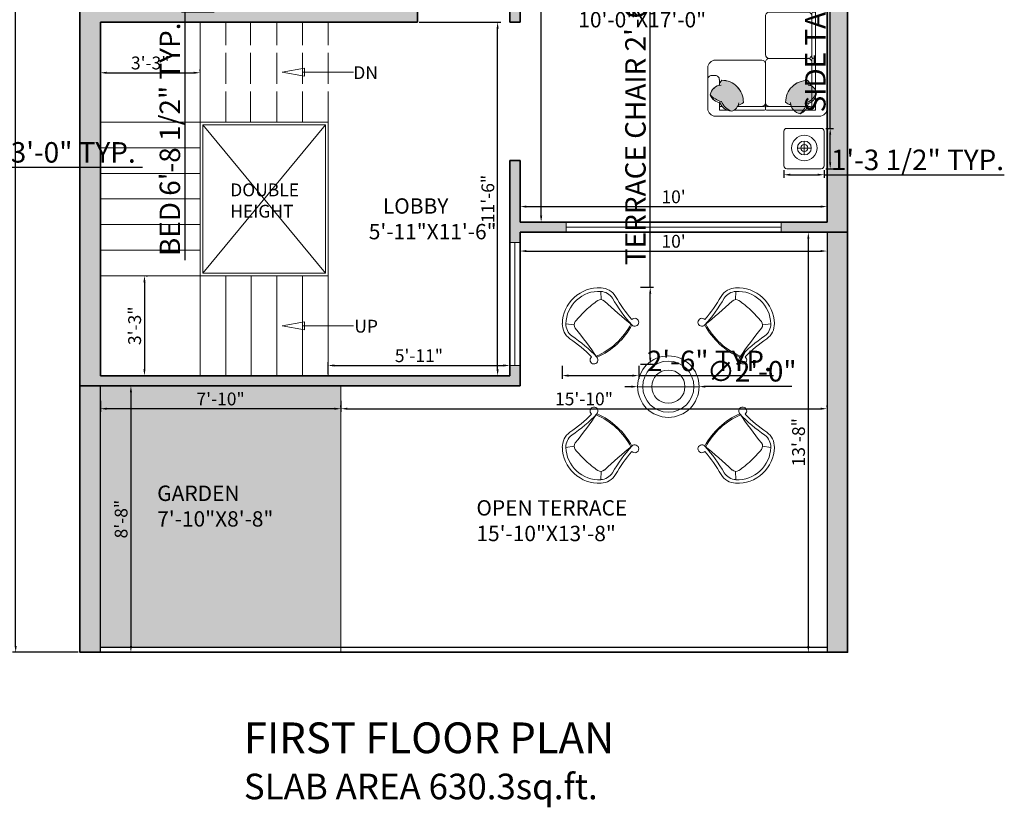
# Model space of a CAD drawing. Units: inches. Extents: x 3259 to 4981, y 1402 to 2026.
# Tile 5 of 11: x 3644 to 4029, y 1415 to 1722. Entities that reach past the tile are written whole.
import ezdxf

# ---------------------------------------------------------------- set-up
doc = ezdxf.new("R2010")
doc.units = ezdxf.units.IN
doc.linetypes.add('ACAD_ISO02W100', pattern=[15, 12, -3])
for name, color, linetype, lineweight in [('A-ANNO-DIMS', 2, 'Continuous', 13), ('A-ANNO-SYMB', 7, 'Continuous', 13), ('A-ANNO-TITL', 7, 'Continuous', 25), ('A-AREA-IDEN', 7, 'Continuous', 18), ('A-DOOR', 3, 'Continuous', 18), ('A-FLOR-STRS', 7, 'Continuous', 18), ('A-FLOR-STRS-OVHD', 8, 'ACAD_ISO02W100', 13), ('A-FURN', 8, 'Continuous', 13), ('A-GLAZ', 4, 'Continuous', 18), ('A-WALL', 7, 'Continuous', 35), ('A-WALL-PATT', 252, 'Continuous', 13), ('A-WALL-PRPT', 7, 'Continuous', 25), ('L-PLNT', 3, 'Continuous', 18)]:
    doc.layers.add(name, color=color, linetype=linetype, lineweight=lineweight)
doc.layers.add('A-WALL-PRPT-PATT', color=9, linetype='Continuous', lineweight=13, true_color=0xc7c8ca)
doc.layers.add('L-PLNT-PATT', color=114, linetype='Continuous', lineweight=13, true_color=0x139b48)
doc.styles.get("Standard").update_dxf_attribs({"font": 'arial.ttf'})
doc.dimstyles.new('ISO-25', dxfattribs={"dimtxt": 8, "dimasz": 2.5, "dimexe": 1.25, "dimexo": 0.625, "dimtad": 1, "dimdec": 1, "dimlunit": 3, "dimtxsty": 'Standard', "dimcen": 2.5, "dimclrd": 4, "dimclre": 4, "dimclrt": 1, "dimadec": 0, "dimazin": 0, "dimtfac": 1, "dimtdec": 1, "dimtmove": 0, "dimatfit": 3, "dimfxl": 1, "dimarcsym": 0})

# ---------------------------------------------------------------- blocks, each defined once
blk = doc.blocks.new('SOFA 1')
at = {"transparency": 33554687}
h = blk.add_hatch(color=256, dxfattribs=at)
h.dxf.hatch_style = 1
h.paths.add_polyline_path([(3769.65, 1307.6, 0.084911), (3767.15, 1309.12, 0.046133), (3766.46, 1311.13), (3759.18, 1311.13, 0.039409), (3758.92, 1310.24, 0.165523), (3756.31, 1309.02, 0.42585), (3767.59, 1297.95, 0.121928), (3769.15, 1300.58, 0.027403), (3769.65, 1300.83)])
h.paths.add_polyline_path([(3765.34, 1313.08), (3760.4, 1313.08, 0.097704), (3759.18, 1311.13), (3766.46, 1311.13, 0.04873)])
h.paths.add_polyline_path([(3763.76, 1314.88, 0.16488), (3760.4, 1313.08), (3765.34, 1313.08, 0.051917)])
h.paths.add_polyline_path([(3771.6, 1305.17, 0.090388), (3769.65, 1307.6), (3769.65, 1300.83, 0.136035), (3771.6, 1302.77)])
h = blk.add_hatch(color=256, dxfattribs=at)
h.dxf.hatch_style = 1
h.paths.add_polyline_path([(3723.52, 1308.63, 0.147724), (3717.76, 1305.24, 0.310469), (3722.42, 1300.4), (3722.42, 1300.25, 0.156703), (3723.62, 1297.8, 0.425821), (3734.69, 1309.08, 0.121928), (3732.05, 1310.63, 0.233216), (3728.6, 1313.59, 0.213835)])
h = blk.add_hatch(color=256, dxfattribs=at)
h.dxf.hatch_style = 1
h.paths.add_polyline_path([(3769.16, 1235.96, 0.122267), (3767.6, 1238.61, 0.425972), (3756.32, 1227.54, 0.165563), (3758.93, 1226.32, 0.309481), (3763.76, 1221.69, 0.002677), (3763.83, 1221.72, 0.146094), (3767.16, 1227.43, 0.212433), (3772.1, 1232.48, 0.235342)])
h = blk.add_hatch(color=256, dxfattribs=at)
h.dxf.hatch_style = 1
h.paths.add_polyline_path([(3769.16, 1225.36, 0.122267), (3767.6, 1228.01, 0.425972), (3756.32, 1216.94, 0.165563), (3758.93, 1215.72, 0.309481), (3763.76, 1211.09, 0.002677), (3763.83, 1211.12, 0.146094), (3767.16, 1216.83, 0.212433), (3772.1, 1221.88, 0.235342)])
for p, q in [((3720.45, 1316.13), (3773.58, 1316.13)), ((3777.51, 1312.19), (3777.51, 1213.72))]:
    blk.add_line(p, q, dxfattribs=at)
for points in [[(3763.76, 1314.88, -0.147724), (3767.15, 1309.12, -0.213355), (3772.1, 1304.05, 0.213355), (3767.15, 1309.12, 0.147724), (3763.76, 1314.88, -0.249545), (3767.86, 1309.77, 0.249545), (3763.77, 1314.89, 0.356779), (3758.8, 1309.23, -0.356779), (3763.76, 1314.88)], [(3717.76, 1305.24, -0.147724), (3723.52, 1308.63, -0.213355), (3728.59, 1313.59, 0.213355), (3723.52, 1308.63, 0.147724), (3717.76, 1305.24, -0.249545), (3722.86, 1309.34, 0.249545), (3717.75, 1305.25, 0.356779), (3723.4, 1300.28, -0.356779), (3717.76, 1305.24)], [(3734.69, 1309.08, -0.425972), (3723.62, 1297.8, -0.165552), (3722.4, 1300.4, 0.165552), (3723.62, 1297.79, 0.425972), (3734.69, 1309.07, 0.121514), (3732.07, 1310.63, -0.121514), (3734.69, 1309.08)], [(3728.58, 1313.6, -0.306333), (3732.42, 1309.31, 0.306333), (3728.58, 1313.6, 0.306674), (3722.72, 1308.89, -0.306674), (3728.58, 1313.6)], [(3767.6, 1297.95, -0.425972), (3756.31, 1309.01, -0.165552), (3758.92, 1310.24, 0.165552), (3756.31, 1309.02, 0.425972), (3767.59, 1297.95, 0.121514), (3769.14, 1300.57, -0.121514), (3767.6, 1297.95)], [(3772.11, 1304.06, -0.306333), (3767.83, 1300.22, 0.306333), (3772.11, 1304.06, 0.306674), (3767.4, 1309.91, -0.306674), (3772.11, 1304.06)], [(3770.44, 1286.63, -0.414214), (3769.66, 1287.4, 0.414214), (3770.44, 1286.63, 0.414214), (3769.66, 1285.83, -0.414214), (3770.44, 1286.63)], [(3748.01, 1262.99, -0.414214), (3746.05, 1264.95, 0.414214), (3748.01, 1262.97, 0.414213), (3746.05, 1261.01, -0.414213), (3748.01, 1262.99)], [(3770.44, 1262.99, -0.414214), (3769.66, 1263.77, 0.414214), (3770.44, 1262.99, 0.414214), (3769.66, 1262.19, -0.414214), (3770.44, 1262.99)], [(3770.83, 1262.97, -0.414214), (3771.61, 1262.19, 0.414214), (3770.83, 1262.99, 0.414214), (3771.61, 1263.77, -0.414214), (3770.83, 1262.97)], [(3748.01, 1239.35, -0.414214), (3746.05, 1241.31, 0.414214), (3748.01, 1239.33, 0.414213), (3746.05, 1237.37, -0.414213), (3748.01, 1239.35)], [(3756.32, 1227.54, -0.425972), (3767.6, 1238.61, -0.121514), (3769.16, 1235.98, 0.121514), (3767.6, 1238.61, 0.425972), (3756.32, 1227.54, 0.165552), (3758.93, 1226.32, -0.165552), (3756.32, 1227.54)], [(3767.7, 1239.33, -0.414214), (3769.66, 1237.37, 0.414214), (3767.7, 1239.35, 0.414214), (3769.66, 1241.31, -0.414214), (3767.7, 1239.33)], [(3770.44, 1239.35, -0.414214), (3769.66, 1240.13, 0.414214), (3770.44, 1239.33, 0.414214), (3769.66, 1238.55, -0.414214), (3770.44, 1239.35)], [(3770.83, 1239.33, -0.414214), (3771.61, 1238.55, 0.414214), (3770.83, 1239.35, 0.414214), (3771.61, 1240.13, -0.414214), (3770.83, 1239.33)], [(3772.1, 1232.5, -0.306674), (3767.41, 1226.64, 0.306674), (3772.1, 1232.5, 0.306333), (3767.84, 1236.34, -0.306333), (3772.1, 1232.5)], [(3763.78, 1221.67, 0.249545), (3767.87, 1226.78, -0.249545), (3763.76, 1221.69, -0.356779), (3758.81, 1227.32, 0.356779), (3763.77, 1221.68, 0.147724), (3767.16, 1227.43, 0.213355), (3772.11, 1232.51, -0.213355), (3767.16, 1227.43, -0.147724), (3763.78, 1221.67)], [(3756.32, 1216.94, -0.200233), (3759.49, 1224.76, 0.200233), (3756.32, 1216.94, 0.165552), (3758.93, 1215.72, -0.165552), (3756.32, 1216.94)], [(3772.1, 1221.9, -0.306674), (3767.41, 1216.04, 0.306674), (3772.1, 1221.9, -0.213355), (3767.16, 1216.83, -0.147724), (3763.77, 1211.08, 0.147724), (3767.15, 1216.83, 0.213355), (3772.1, 1221.9)], [(3763.76, 1211.09, -0.356779), (3758.81, 1216.72, 0.356779), (3763.76, 1211.09, 0.249545), (3767.87, 1216.18, -0.249545), (3763.76, 1211.09)]]:
    blk.add_lwpolyline(points, format="xyb", dxfattribs=at)
for points in [[(3716.51, 1312.2), (3716.51, 1291.44)], [(3722.42, 1313.08), (3722.42, 1309.23), (3722.42, 1313.08), (3726.57, 1313.08)], [(3723.21, 1311.13), (3723.93, 1311.13)], [(3729.85, 1313.08), (3745.25, 1313.08)], [(3731.82, 1311.13), (3745.25, 1311.13)], [(3746.01, 1312.3), (3746.01, 1288.55)], [(3746.01, 1310.97), (3746.01, 1311.36)], [(3768.11, 1313.08), (3746.78, 1313.08)], [(3768.87, 1311.13), (3746.78, 1311.13)], [(3771.6, 1313.08), (3767.75, 1313.08), (3771.6, 1313.08), (3771.6, 1308.93)], [(3769.66, 1287.39), (3769.65, 1312.3)], [(3769.65, 1309.43), (3769.65, 1308.71)], [(3771.6, 1313.08), (3771.61, 1233.74)], [(3746.01, 1288.54), (3746.01, 1308.23)], [(3722.42, 1300.39), (3722.42, 1297.33)], [(3720.45, 1295.38), (3718.48, 1295.38)], [(3720.45, 1287.5), (3744.09, 1287.5)], [(3746.02, 1284.63), (3746.02, 1264.94)], [(3747.99, 1286.6), (3767.69, 1286.6)], [(3769.66, 1263.75), (3769.66, 1285.81)], [(3769.66, 1277.18), (3769.66, 1263.75)], [(3746.02, 1260.99), (3746.02, 1241.3)], [(3747.99, 1262.97), (3767.69, 1262.97)], [(3769.66, 1240.12), (3769.66, 1262.18)], [(3770.43, 1262.97), (3770.82, 1262.97)], [(3747.99, 1239.33), (3767.69, 1239.33)], [(3769.66, 1235.71), (3769.66, 1238.54)], [(3770.43, 1239.33), (3770.82, 1239.33)], [(3746.02, 1237.36), (3746.02, 1213.74)], [(3771.61, 1223.14), (3771.61, 1230.47)], [(3769.66, 1225.11), (3769.66, 1227.82)], [(3767.76, 1215.72), (3771.61, 1215.72), (3771.61, 1219.84), (3771.61, 1215.72)], [(3753.91, 1211.77), (3753.91, 1213.74)], [(3755.86, 1215.72), (3758.92, 1215.72)], [(3769.66, 1216.5), (3769.66, 1217.22)], [(3749.97, 1209.8), (3773.58, 1209.8)]]:
    blk.add_lwpolyline(points, close=True, dxfattribs=at)
for points in [[(3722.42, 1311.91, 0.414214), (3723.2, 1311.13, -0.414214)], [(3770.43, 1313.08, 0.414214), (3769.65, 1312.3, -0.414214)], [(3771.6, 1312.3, 0.414214), (3770.82, 1313.08, -0.414214)], [(3716.51, 1297.34, 0.414214), (3718.47, 1295.38, -0.414214)], [(3720.44, 1295.38, 0.414214), (3722.4, 1297.34, -0.414214)], [(3716.51, 1291.45, 0.414212), (3720.44, 1287.52, -0.414212)], [(3746.03, 1288.56, 0.414214), (3747.99, 1286.6, 0.414213), (3746.03, 1284.64, -0.414213), (3747.99, 1286.6, -0.414214)], [(3769.66, 1284.64, 0.414214), (3767.7, 1286.6, 0.414214), (3769.66, 1288.56, -0.414214), (3767.7, 1286.6, -0.414214)], [(3769.66, 1261.01, 0.414214), (3767.7, 1262.97, 0.414214), (3769.66, 1264.93, -0.414214), (3767.7, 1262.97, -0.414214)], [(3772.13, 1221.9, 0.306333), (3767.84, 1225.74, -0.306333)], [(3769.16, 1225.36, 0.071861), (3768.39, 1227.01, -0.071861)], [(3746.05, 1213.76, 0.414212), (3749.98, 1209.82, -0.414212)], [(3755.87, 1215.72, 0.414214), (3753.91, 1213.76, -0.414214)], [(3769.66, 1216.52, 0.414214), (3770.44, 1215.74, -0.414214)], [(3770.83, 1215.74, 0.414214), (3771.61, 1216.52, -0.414214)], [(3755.87, 1209.8, -0.414214), (3753.91, 1211.76, 0.414214)]]:
    blk.add_lwpolyline(points, format="xyb", close=True, dxfattribs=at)
for centre, radius, start, end in [((3720.44, 1312.2), 3.93, 90.0002, 179.9998), ((3720.44, 1312.19), 3.94, 89.9158, 179.9154), ((3773.58, 1312.2), 3.93, 0.0002, 89.9998), ((3773.57, 1312.19), 3.94, 359.9158, 89.9154), ((3744.09, 1309.21), 1.92, 358.766, 90.5111), ((3745.22, 1312.29), 0.789, 0.8425, 90.8425), ((3745.24, 1311.91), 0.777, 270, 0), ((3745.24, 1311.91), 0.777, 270, 0), ((3746.8, 1312.29), 0.789, 89.1575, 179.1575), ((3746.79, 1311.91), 0.777, 180, 270), ((3746.79, 1311.91), 0.777, 180, 270), ((3747.93, 1309.21), 1.92, 89.4889, 181.234), ((3768.87, 1312.3), 0.777, 360, 90), ((3768.87, 1311.91), 0.777, 270, 0), ((3744.08, 1289.48), 1.96, 270, 360), ((3744.08, 1289.48), 1.96, 270, 360), ((3773.58, 1213.73), 3.93, 270.0002, 359.9998), ((3773.59, 1213.73), 3.93, 269.9156, 359.9152)]:
    blk.add_arc(centre, radius, start, end, dxfattribs=at)
blk = doc.blocks.new('table-31')
at = {"color": 0, "linetype": 'ByBlock'}
for p, q in [((-0.2031, 0.1666), (-0.2031, -0.1763)), ((0.1683, 0.1952), (-0.1746, 0.1952)), ((0.1969, 0.1666), (0.1969, -0.1763)), ((-0.0689, 0), (0.0689, 0)), ((0, -0.0689), (0, 0.0689)), ((0.1683, -0.2048), (-0.1746, -0.2048))]:
    blk.add_line(p, q, dxfattribs=at)
for radius in [0.1261, 0.0689, 0.0353]:
    blk.add_circle((0, 0), radius, dxfattribs=at)
for centre, start, end in [((-0.1746, 0.1666), 90, 180), ((0.1683, 0.1666), 0, 90), ((-0.1746, -0.1763), 180, 270), ((0.1683, -0.1763), 270, 0)]:
    blk.add_arc(centre, 0.0286, start, end, dxfattribs=at)
blk = doc.blocks.new('*D49')
at = {"layer": 'A-ANNO-DIMS', "color": 0, "lineweight": -2, "transparency": 16777216}
for p, q in [((3675.66, 1573.27), (3675.66, 1568.97)), ((3767.16, 1570.22), (3678.16, 1570.22)), ((3769.66, 1573.27), (3769.66, 1568.97))]:
    blk.add_line(p, q, dxfattribs=at)
at = {"layer": 'A-ANNO-DIMS', "color": 0, "transparency": 16777216}
for points in [[(3678.16, 1570.63), (3678.16, 1569.8), (3675.66, 1570.22)], [(3767.16, 1570.63), (3767.16, 1569.8), (3769.66, 1570.22)]]:
    blk.add_solid(points, dxfattribs=at)
at = {"layer": 'Defpoints', "color": 0, "transparency": 16777216}
for p in [(3675.66, 1573.89), (3769.66, 1573.89), (3675.66, 1570.22)]:
    blk.add_point(p, dxfattribs=at)
at = {"layer": 'A-ANNO-DIMS', "color": 0, "transparency": 16777216, "insert": (3722.66, 1573.4), "char_height": 5, "attachment_point": 5}
blk.add_mtext('7\'-10"', dxfattribs=at)
blk = doc.blocks.new('*D50')
at = {"layer": 'A-ANNO-DIMS', "color": 0, "lineweight": -2, "transparency": 16777216}
for p, q in [((3686.25, 1579.12), (3688.85, 1579.12)), ((3687.6, 1576.62), (3687.6, 1477.62)), ((3686.25, 1475.12), (3688.85, 1475.12))]:
    blk.add_line(p, q, dxfattribs=at)
at = {"layer": 'A-ANNO-DIMS', "color": 0, "transparency": 16777216}
for points in [[(3687.18, 1576.62), (3688.02, 1576.62), (3687.6, 1579.12)], [(3687.18, 1477.62), (3688.02, 1477.62), (3687.6, 1475.12)]]:
    blk.add_solid(points, dxfattribs=at)
at = {"layer": 'Defpoints', "color": 0, "transparency": 16777216}
for p in [(3685.62, 1579.12), (3685.62, 1475.12), (3687.6, 1475.12)]:
    blk.add_point(p, dxfattribs=at)
at = {"layer": 'A-ANNO-DIMS', "color": 0, "transparency": 16777216, "insert": (3684.42, 1527.12), "char_height": 5, "attachment_point": 5, "rotation": 90}
blk.add_mtext('8\'-8"', dxfattribs=at)
blk = doc.blocks.new('*D51')
at = {"layer": 'A-ANNO-DIMS', "color": 0, "lineweight": -2, "transparency": 16777216}
for p, q in [((3769.66, 1570.84), (3769.66, 1571.47)), ((3772.16, 1570.22), (3957.16, 1570.22)), ((3959.66, 1570.84), (3959.66, 1571.47))]:
    blk.add_line(p, q, dxfattribs=at)
at = {"layer": 'A-ANNO-DIMS', "color": 0, "transparency": 16777216}
for points in [[(3772.16, 1570.63), (3772.16, 1569.8), (3769.66, 1570.22)], [(3957.16, 1570.63), (3957.16, 1569.8), (3959.66, 1570.22)]]:
    blk.add_solid(points, dxfattribs=at)
at = {"layer": 'Defpoints', "color": 0, "transparency": 16777216}
for p in [(3769.66, 1570.22), (3959.66, 1570.22), (3959.66, 1570.22)]:
    blk.add_point(p, dxfattribs=at)
at = {"layer": 'A-ANNO-DIMS', "color": 0, "transparency": 16777216, "insert": (3864.66, 1573.4), "char_height": 5, "attachment_point": 5}
blk.add_mtext('15\'-10"', dxfattribs=at)
blk = doc.blocks.new('*D52')
at = {"layer": 'A-ANNO-DIMS', "color": 0, "lineweight": -2, "transparency": 16777216}
for p, q in [((3959.04, 1639.12), (3951.08, 1639.12)), ((3952.33, 1477.62), (3952.33, 1636.62)), ((3959.04, 1475.12), (3951.08, 1475.12))]:
    blk.add_line(p, q, dxfattribs=at)
at = {"layer": 'A-ANNO-DIMS', "color": 0, "transparency": 16777216}
for points in [[(3951.91, 1636.62), (3952.74, 1636.62), (3952.33, 1639.12)], [(3951.91, 1477.62), (3952.74, 1477.62), (3952.33, 1475.12)]]:
    blk.add_solid(points, dxfattribs=at)
at = {"layer": 'Defpoints', "color": 0, "transparency": 16777216}
for p in [(3952.33, 1639.12), (3959.66, 1639.12), (3959.66, 1475.12)]:
    blk.add_point(p, dxfattribs=at)
at = {"layer": 'A-ANNO-DIMS', "color": 0, "transparency": 16777216, "insert": (3949.15, 1557.12), "char_height": 5, "attachment_point": 5, "rotation": 90}
blk.add_mtext('13\'-8"', dxfattribs=at)
blk = doc.blocks.new('*D53')
at = {"layer": 'A-ANNO-DIMS', "color": 0, "lineweight": -2, "transparency": 16777216}
for p, q in [((3764.66, 1583.74), (3764.66, 1588.35)), ((3767.16, 1587.1), (3833.16, 1587.1)), ((3835.66, 1583.74), (3835.66, 1588.35))]:
    blk.add_line(p, q, dxfattribs=at)
at = {"layer": 'A-ANNO-DIMS', "color": 0, "transparency": 16777216}
for points in [[(3767.16, 1587.52), (3767.16, 1586.68), (3764.66, 1587.1)], [(3833.16, 1587.52), (3833.16, 1586.68), (3835.66, 1587.1)]]:
    blk.add_solid(points, dxfattribs=at)
at = {"layer": 'Defpoints', "color": 0, "transparency": 16777216}
for p in [(3835.66, 1587.1), (3764.66, 1583.12), (3835.66, 1583.12)]:
    blk.add_point(p, dxfattribs=at)
at = {"layer": 'A-ANNO-DIMS', "color": 0, "transparency": 16777216, "insert": (3800.16, 1590.28), "char_height": 5, "attachment_point": 5}
blk.add_mtext('5\'-11"', dxfattribs=at)
blk = doc.blocks.new('*D54')
at = {"layer": 'A-ANNO-DIMS', "color": 0, "lineweight": -2, "transparency": 16777216}
for p, q in [((3800.29, 1721.12), (3832.16, 1721.12)), ((3830.91, 1585.62), (3830.91, 1718.62)), ((3835.04, 1583.12), (3829.66, 1583.12))]:
    blk.add_line(p, q, dxfattribs=at)
at = {"layer": 'A-ANNO-DIMS', "color": 0, "transparency": 16777216}
for points in [[(3830.49, 1718.62), (3831.32, 1718.62), (3830.91, 1721.12)], [(3830.49, 1585.62), (3831.32, 1585.62), (3830.91, 1583.12)]]:
    blk.add_solid(points, dxfattribs=at)
at = {"layer": 'Defpoints', "color": 0, "transparency": 16777216}
for p in [(3799.66, 1721.12), (3830.91, 1721.12), (3835.66, 1583.12)]:
    blk.add_point(p, dxfattribs=at)
at = {"layer": 'A-ANNO-DIMS', "color": 0, "transparency": 16777216, "insert": (3827.73, 1652.12), "char_height": 5, "attachment_point": 5, "rotation": 90}
blk.add_mtext('11\'-6"', dxfattribs=at)
blk = doc.blocks.new('*D55')
at = {"layer": 'A-ANNO-DIMS', "color": 0, "lineweight": -2, "transparency": 16777216}
for p, q in [((3839.66, 1643.74), (3839.66, 1650.4)), ((3842.16, 1649.15), (3957.16, 1649.15)), ((3959.66, 1643.74), (3959.66, 1650.4))]:
    blk.add_line(p, q, dxfattribs=at)
at = {"layer": 'A-ANNO-DIMS', "color": 0, "transparency": 16777216}
for points in [[(3842.16, 1649.56), (3842.16, 1648.73), (3839.66, 1649.15)], [(3957.16, 1649.56), (3957.16, 1648.73), (3959.66, 1649.15)]]:
    blk.add_solid(points, dxfattribs=at)
at = {"layer": 'Defpoints', "color": 0, "transparency": 16777216}
for p in [(3959.66, 1649.15), (3839.66, 1643.12), (3959.66, 1643.12)]:
    blk.add_point(p, dxfattribs=at)
at = {"layer": 'A-ANNO-DIMS', "color": 0, "transparency": 16777216, "insert": (3899.66, 1652.32), "char_height": 5, "attachment_point": 5}
blk.add_mtext("10'", dxfattribs=at)
blk = doc.blocks.new('*D56')
at = {"layer": 'A-ANNO-DIMS', "color": 0, "lineweight": -2, "transparency": 16777216}
for p, q in [((3840.29, 1847.12), (3849.16, 1847.12)), ((3847.91, 1645.62), (3847.91, 1844.62)), ((3840.29, 1643.12), (3849.16, 1643.12))]:
    blk.add_line(p, q, dxfattribs=at)
at = {"layer": 'A-ANNO-DIMS', "color": 0, "transparency": 16777216}
for points in [[(3847.49, 1844.62), (3848.33, 1844.62), (3847.91, 1847.12)], [(3847.49, 1645.62), (3848.33, 1645.62), (3847.91, 1643.12)]]:
    blk.add_solid(points, dxfattribs=at)
at = {"layer": 'Defpoints', "color": 0, "transparency": 16777216}
for p in [(3839.66, 1847.12), (3847.91, 1847.12), (3839.66, 1643.12)]:
    blk.add_point(p, dxfattribs=at)
at = {"layer": 'A-ANNO-DIMS', "color": 0, "transparency": 16777216, "insert": (3844.77, 1745.12), "char_height": 5, "attachment_point": 5, "rotation": 90}
blk.add_mtext("17'", dxfattribs=at)
blk = doc.blocks.new('*D57')
at = {"layer": 'A-ANNO-DIMS', "color": 0, "lineweight": -2, "transparency": 16777216}
for p, q in [((3675.66, 1702.02), (3675.66, 1702.65)), ((3678.16, 1701.4), (3712.16, 1701.4)), ((3714.66, 1702.02), (3714.66, 1702.65))]:
    blk.add_line(p, q, dxfattribs=at)
at = {"layer": 'A-ANNO-DIMS', "color": 0, "transparency": 16777216}
for points in [[(3678.16, 1701.81), (3678.16, 1700.98), (3675.66, 1701.4)], [(3712.16, 1701.81), (3712.16, 1700.98), (3714.66, 1701.4)]]:
    blk.add_solid(points, dxfattribs=at)
at = {"layer": 'Defpoints', "color": 0, "transparency": 16777216}
for p in [(3675.66, 1701.4), (3714.66, 1701.4), (3714.66, 1701.4)]:
    blk.add_point(p, dxfattribs=at)
at = {"layer": 'A-ANNO-DIMS', "color": 0, "transparency": 16777216, "insert": (3695.16, 1704.57), "char_height": 5, "attachment_point": 5}
blk.add_mtext('3\'-3"', dxfattribs=at)
blk = doc.blocks.new('*D58')
at = {"layer": 'A-ANNO-DIMS', "color": 0, "lineweight": -2, "transparency": 16777216}
for p, q in [((3693.52, 1622.12), (3694.14, 1622.12)), ((3692.89, 1619.62), (3692.89, 1585.62)), ((3693.52, 1583.12), (3694.14, 1583.12))]:
    blk.add_line(p, q, dxfattribs=at)
at = {"layer": 'A-ANNO-DIMS', "color": 0, "transparency": 16777216}
for points in [[(3692.48, 1619.62), (3693.31, 1619.62), (3692.89, 1622.12)], [(3692.48, 1585.62), (3693.31, 1585.62), (3692.89, 1583.12)]]:
    blk.add_solid(points, dxfattribs=at)
at = {"layer": 'Defpoints', "color": 0, "transparency": 16777216}
for p in [(3692.89, 1622.12), (3692.89, 1583.12), (3692.89, 1583.12)]:
    blk.add_point(p, dxfattribs=at)
at = {"layer": 'A-ANNO-DIMS', "color": 0, "transparency": 16777216, "insert": (3689.71, 1602.62), "char_height": 5, "attachment_point": 5, "rotation": 90}
blk.add_mtext('3\'-3"', dxfattribs=at)
blk = doc.blocks.new('*D60')
at = {"layer": 'A-ANNO-DIMS', "color": 0, "lineweight": -2, "transparency": 16777216}
for p, q in [((3839.66, 1638.49), (3839.66, 1630.53)), ((3959.66, 1638.49), (3959.66, 1630.53)), ((3842.16, 1631.78), (3957.16, 1631.78))]:
    blk.add_line(p, q, dxfattribs=at)
at = {"layer": 'A-ANNO-DIMS', "color": 0, "transparency": 16777216}
for points in [[(3842.16, 1632.2), (3842.16, 1631.37), (3839.66, 1631.78)], [(3957.16, 1632.2), (3957.16, 1631.37), (3959.66, 1631.78)]]:
    blk.add_solid(points, dxfattribs=at)
at = {"layer": 'Defpoints', "color": 0, "transparency": 16777216}
for p in [(3839.66, 1639.12), (3959.66, 1639.12), (3959.66, 1631.78)]:
    blk.add_point(p, dxfattribs=at)
at = {"layer": 'A-ANNO-DIMS', "color": 0, "transparency": 16777216, "insert": (3899.66, 1634.96), "char_height": 5, "attachment_point": 5}
blk.add_mtext("10'", dxfattribs=at)
blk = doc.blocks.new('A$C16EC238A')
for p, q in [((490, 810), (485, 914)), ((148, 493), (45, 507))]:
    blk.add_line(p, q)
for centre, radius, start, end in [((464, 496), 464, 87.0599, 178.502), ((464, 496), 419, 87.0599, 178.502), ((476, 730), 184, 31.9256, 87.0599), ((476, 730), 229, 31.9256, 87.0599), ((1209, -303), 1339, 124.646, 132.9725), ((486, 744), 66, 46.736, 125.0291), ((4628, 5145), 5977, 226.736, 231.1302), ((2169, 1687), 1760, 209.219, 222.7724), ((2169, 1687), 1715, 209.219, 221.1077), ((1301, -402), 1474, 132.9725, 140.5328), ((229, 502), 229, 178.502, 233.6363), ((229, 502), 184, 178.502, 233.6363), ((214, 493), 66, 140.5328, 218.8259), ((62, 930), 910, 293.6787, 331.8832), ((913, 525), 50, 222.7809, 137.6785), ((-4494, -3296), 5977, 34.4317, 38.8259), ((62, 930), 925, 293.8563, 331.7056), ((-856, -1112), 1715, 44.4541, 56.3429), ((-856, -1112), 1760, 42.7895, 56.3429), ((399, 50), 50, 127.8834, 42.7809)]:
    blk.add_arc(centre, radius, start, end)
blk = doc.blocks.new('STAIR-WELL-50x60')
for p, q in [((1, 59), (49, 1)), ((1, 1), (49, 59))]:
    blk.add_line(p, q)
for points in [[(50, 60), (0, 60), (0, 0), (50, 0)], [(49, 59), (1, 59), (1, 1), (49, 1)]]:
    blk.add_lwpolyline(points, close=True)
blk = doc.blocks.new('STAIR-DIRECTION')
blk.add_line((7.93, 1.55), (27.85, 1.55))
blk.add_lwpolyline([(0, 1.55), (8.64, 3.11), (8.64, 0)], close=True)
blk = doc.blocks.new('*D152')
at = {"layer": 'A-ANNO-DIMS', "color": 4, "lineweight": -2, "transparency": 16777216}
for p, q in [((3890.55, 1617.63), (3890.55, 1764.73)), ((3886.68, 1617.63), (3891.8, 1617.63)), ((3890.55, 1590.15), (3890.55, 1615.13)), ((3886.68, 1587.65), (3891.8, 1587.65))]:
    blk.add_line(p, q, dxfattribs=at)
at = {"layer": 'A-ANNO-DIMS', "color": 4, "transparency": 16777216}
for points in [[(3890.13, 1615.13), (3890.96, 1615.13), (3890.55, 1617.63)], [(3890.13, 1590.15), (3890.96, 1590.15), (3890.55, 1587.65)]]:
    blk.add_solid(points, dxfattribs=at)
at = {"layer": 'Defpoints', "color": 0, "transparency": 16777216}
for p in [(3886.05, 1617.63), (3890.55, 1617.63), (3886.05, 1587.65)]:
    blk.add_point(p, dxfattribs=at)
at = {"layer": 'A-ANNO-DIMS', "color": 1, "transparency": 16777216, "insert": (3885.79, 1692.43), "char_height": 8, "attachment_point": 5, "rotation": 90}
blk.add_mtext('TERRACE CHAIR 2\'-6" TYP.', dxfattribs=at)
blk = doc.blocks.new('*D153')
at = {"layer": 'A-ANNO-DIMS', "color": 4, "lineweight": -2, "transparency": 16777216}
for p, q in [((3856.13, 1587.02), (3856.13, 1581.9)), ((3886.05, 1587.02), (3886.05, 1581.9)), ((3858.63, 1583.15), (3883.55, 1583.15)), ((3886.05, 1583.15), (3938.7, 1583.15))]:
    blk.add_line(p, q, dxfattribs=at)
at = {"layer": 'A-ANNO-DIMS', "color": 4, "transparency": 16777216}
for points in [[(3858.63, 1583.57), (3858.63, 1582.73), (3856.13, 1583.15)], [(3883.55, 1583.57), (3883.55, 1582.73), (3886.05, 1583.15)]]:
    blk.add_solid(points, dxfattribs=at)
at = {"layer": 'Defpoints', "color": 0, "transparency": 16777216}
for p in [(3856.13, 1587.65), (3886.05, 1587.65), (3886.05, 1583.15)]:
    blk.add_point(p, dxfattribs=at)
at = {"layer": 'A-ANNO-DIMS', "color": 1, "transparency": 16777216, "insert": (3913.63, 1587.86), "char_height": 8, "attachment_point": 5}
blk.add_mtext('2\'-6" TYP.', dxfattribs=at)
blk = doc.blocks.new('*D158')
at = {"layer": 'A-ANNO-DIMS', "color": 4, "lineweight": -2, "transparency": 16777216}
for p, q in [((3720.1, 1805.78), (3707.38, 1805.78)), ((3708.63, 1803.28), (3708.63, 1727.62)), ((3720.1, 1725.12), (3707.38, 1725.12)), ((3708.63, 1725.12), (3708.63, 1628.23))]:
    blk.add_line(p, q, dxfattribs=at)
at = {"layer": 'A-ANNO-DIMS', "color": 4, "transparency": 16777216}
for points in [[(3708.21, 1803.28), (3709.04, 1803.28), (3708.63, 1805.78)], [(3708.21, 1727.62), (3709.04, 1727.62), (3708.63, 1725.12)]]:
    blk.add_solid(points, dxfattribs=at)
at = {"layer": 'Defpoints', "color": 0, "transparency": 16777216}
for p in [(3720.73, 1805.78), (3708.63, 1725.12), (3720.73, 1725.12)]:
    blk.add_point(p, dxfattribs=at)
at = {"layer": 'A-ANNO-DIMS', "color": 1, "transparency": 16777216, "insert": (3703.87, 1675.42), "char_height": 8, "attachment_point": 5, "rotation": 90}
blk.add_mtext('BED 6\'-8 1/2" TYP.', dxfattribs=at)
blk = doc.blocks.new('*D160')
at = {"layer": 'A-ANNO-DIMS', "color": 4, "lineweight": -2, "transparency": 16777216}
for p, q in [((3960.87, 1679.69), (3960.87, 1818.51)), ((3959.13, 1679.69), (3962.12, 1679.69)), ((3960.87, 1666.44), (3960.87, 1677.19)), ((3959.13, 1663.94), (3962.12, 1663.94))]:
    blk.add_line(p, q, dxfattribs=at)
at = {"layer": 'A-ANNO-DIMS', "color": 4, "transparency": 16777216}
for points in [[(3960.45, 1677.19), (3961.28, 1677.19), (3960.87, 1679.69)], [(3960.45, 1666.44), (3961.28, 1666.44), (3960.87, 1663.94)]]:
    blk.add_solid(points, dxfattribs=at)
at = {"layer": 'Defpoints', "color": 0, "transparency": 16777216}
for p in [(3958.51, 1679.69), (3960.87, 1679.69), (3958.51, 1663.94)]:
    blk.add_point(p, dxfattribs=at)
at = {"layer": 'A-ANNO-DIMS', "color": 1, "transparency": 16777216, "insert": (3956.1, 1750.35), "char_height": 8, "attachment_point": 5, "rotation": 90}
blk.add_mtext('SIDE TABLE 1\'-3 1/2" TYP.', dxfattribs=at)
blk = doc.blocks.new('*D161')
at = {"layer": 'A-ANNO-DIMS', "color": 4, "lineweight": -2, "transparency": 16777216}
for p, q in [((3942.76, 1663.32), (3942.76, 1660.33)), ((3958.51, 1663.32), (3958.51, 1660.33)), ((3945.26, 1661.58), (3956.01, 1661.58)), ((3958.51, 1661.58), (4028.91, 1661.58))]:
    blk.add_line(p, q, dxfattribs=at)
at = {"layer": 'A-ANNO-DIMS', "color": 4, "transparency": 16777216}
for points in [[(3945.26, 1662), (3945.26, 1661.16), (3942.76, 1661.58)], [(3956.01, 1662), (3956.01, 1661.16), (3958.51, 1661.58)]]:
    blk.add_solid(points, dxfattribs=at)
at = {"layer": 'Defpoints', "color": 0, "transparency": 16777216}
for p in [(3942.76, 1663.94), (3958.51, 1663.94), (3958.51, 1661.58)]:
    blk.add_point(p, dxfattribs=at)
at = {"layer": 'A-ANNO-DIMS', "color": 1, "transparency": 16777216, "insert": (3994.96, 1666.35), "char_height": 8, "attachment_point": 5}
blk.add_mtext('1\'-3 1/2" TYP.', dxfattribs=at)
blk = doc.blocks.new('*D176')
at = {"layer": 'A-ANNO-DIMS', "color": 4, "lineweight": -2, "transparency": 16777216}
for p, q in [((3551.16, 1659.74), (3551.16, 1665.77)), ((3553.66, 1664.52), (3584.66, 1664.52)), ((3587.16, 1659.74), (3587.16, 1665.77)), ((3587.16, 1664.52), (3692.15, 1664.52))]:
    blk.add_line(p, q, dxfattribs=at)
at = {"layer": 'A-ANNO-DIMS', "color": 4, "transparency": 16777216}
for points in [[(3553.66, 1664.93), (3553.66, 1664.1), (3551.16, 1664.52)], [(3584.66, 1664.93), (3584.66, 1664.1), (3587.16, 1664.52)]]:
    blk.add_solid(points, dxfattribs=at)
at = {"layer": 'Defpoints', "color": 0, "transparency": 16777216}
for p in [(3587.16, 1664.52), (3551.16, 1659.12), (3587.16, 1659.12)]:
    blk.add_point(p, dxfattribs=at)
at = {"layer": 'A-ANNO-DIMS', "color": 1, "transparency": 16777216, "insert": (3640.91, 1669.28), "char_height": 8, "attachment_point": 5}
blk.add_mtext('WINDOW 3\'-0" TYP.', dxfattribs=at)
blk = doc.blocks.new('*D187')
at = {"layer": 'A-ANNO-DIMS', "color": 4, "lineweight": -2, "transparency": 16777216}
for p, q in [((3667.04, 1907.12), (3641.31, 1907.12)), ((3642.56, 1477.62), (3642.56, 1904.62)), ((3667.04, 1475.12), (3641.31, 1475.12))]:
    blk.add_line(p, q, dxfattribs=at)
at = {"layer": 'A-ANNO-DIMS', "color": 4, "transparency": 16777216}
for points in [[(3642.15, 1904.62), (3642.98, 1904.62), (3642.56, 1907.12)], [(3642.15, 1477.62), (3642.98, 1477.62), (3642.56, 1475.12)]]:
    blk.add_solid(points, dxfattribs=at)
at = {"layer": 'Defpoints', "color": 0, "transparency": 16777216}
for p in [(3642.56, 1907.12), (3667.66, 1907.12), (3667.66, 1475.12)]:
    blk.add_point(p, dxfattribs=at)
at = {"layer": 'A-ANNO-DIMS', "color": 1, "transparency": 16777216, "insert": (3637.85, 1691.12), "char_height": 8, "attachment_point": 5, "rotation": 90}
blk.add_mtext('36\'-0"', dxfattribs=at)
blk = doc.blocks.new('*D201')
at = {"layer": 'A-ANNO-DIMS', "color": 4, "lineweight": -2, "transparency": 16777216}
for p, q in [((3883.12, 1578.83), (3880.62, 1578.83)), ((3885.62, 1578.83), (3909.62, 1578.85)), ((3945.84, 1578.88), (3912.12, 1578.85))]:
    blk.add_line(p, q, dxfattribs=at)
at = {"layer": 'A-ANNO-DIMS', "color": 4, "transparency": 16777216}
for points in [[(3883.12, 1579.25), (3883.12, 1578.41), (3885.62, 1578.83)], [(3912.12, 1579.27), (3912.12, 1578.44), (3909.62, 1578.85)]]:
    blk.add_solid(points, dxfattribs=at)
at = {"layer": 'Defpoints', "color": 0, "transparency": 16777216}
for p in [(3885.62, 1578.83), (3909.62, 1578.85)]:
    blk.add_point(p, dxfattribs=at)
at = {"layer": 'A-ANNO-DIMS', "color": 1, "transparency": 16777216, "insert": (3930.22, 1583.8), "char_height": 8, "attachment_point": 5, "rotation": 0.0402}
blk.add_mtext('∅2\'-0"', dxfattribs=at)

msp = doc.modelspace()

# ---------------------------------------------------------------- hatches: boundary and pattern name
at = {"layer": 'A-WALL-PATT'}
h = msp.add_hatch(color=256, dxfattribs=at)
h.dxf.hatch_style = 1
h.paths.add_polyline_path([(3839.66, 1851.12), (3835.66, 1851.12), (3835.66, 1721.12), (3839.66, 1721.12), (3839.66, 1777.43), (3839.65, 1777.43), (3839.65, 1777.47), (3839.66, 1777.47), (3839.66, 1781.5), (3839.66, 1781.5), (3839.66, 1781.55)], flags=17)
h.paths.add_polyline_path([(3799.66, 1863.12), (3795.66, 1863.12), (3795.66, 1851.12), (3711.66, 1851.12), (3711.66, 1847.12), (3749.49, 1847.12), (3749.49, 1847.13), (3749.54, 1847.13), (3749.54, 1847.12), (3753.57, 1847.12), (3753.57, 1847.12), (3753.61, 1847.12), (3799.66, 1847.12)], flags=17)
h.paths.add_polyline_path([(3875.66, 1863.12), (3871.66, 1863.12), (3871.66, 1847.12), (3875.66, 1847.12)], flags=17)
h.paths.add_polyline_path([(3967.66, 1907.12), (3667.66, 1907.12), (3667.66, 1579.12), (3839.66, 1579.12), (3839.66, 1587.12), (3835.66, 1587.12), (3835.66, 1583.12), (3675.66, 1583.12), (3675.66, 1721.12), (3799.66, 1721.12), (3799.66, 1725.12), (3675.66, 1725.12), (3675.66, 1899.12), (3711.66, 1899.12), (3711.66, 1881.12), (3715.66, 1881.12), (3715.66, 1899.12), (3795.66, 1899.12), (3795.66, 1887.12), (3799.66, 1887.12), (3799.66, 1899.12), (3871.66, 1899.12), (3871.66, 1887.12), (3875.66, 1887.12), (3875.66, 1899.12), (3959.66, 1899.12), (3959.66, 1851.12), (3905.66, 1851.12), (3905.66, 1847.12), (3959.66, 1847.12), (3959.66, 1643.12), (3941.66, 1643.12), (3941.66, 1639.12), (3967.66, 1639.12)])
h.paths.add_polyline_path([(3839.66, 1667.12), (3835.66, 1667.12), (3835.66, 1635.12), (3839.66, 1635.12), (3839.66, 1639.12), (3857.66, 1639.12), (3857.66, 1643.12), (3839.66, 1643.12)], flags=17)
at = {"layer": 'A-WALL-PRPT-PATT'}
h = msp.add_hatch(color=256, dxfattribs=at)
h.dxf.hatch_style = 1
h.paths.add_polyline_path([(3967.66, 1639.12), (3959.66, 1639.12), (3959.66, 1475.12), (3967.66, 1475.12)])
h.paths.add_polyline_path([(3675.66, 1579.12), (3667.66, 1579.12), (3667.66, 1475.12), (3675.66, 1475.12)])
at = {"layer": 'L-PLNT-PATT'}
h = msp.add_hatch(color=256, dxfattribs=at)
h.dxf.hatch_style = 1
h.paths.add_polyline_path([(3769.66, 1579.12), (3675.66, 1579.12), (3675.66, 1477.12), (3769.66, 1477.12)])
h.paths.add_polyline_path([(3695.94, 1520.8), (3742.62, 1520.8), (3742.62, 1543.19), (3695.94, 1543.19)], flags=24)

# ---------------------------------------------------------------- linework, layer by layer
at = {"layer": 'A-DOOR'}
for p, q in [((3835.66, 1635.12), (3839.66, 1635.12)), ((3837.66, 1635.12), (3837.66, 1587.12)), ((3839.66, 1587.12), (3835.66, 1587.12))]:
    msp.add_line(p, q, dxfattribs=at)
at = {"layer": 'A-FLOR-STRS'}
for p, q in [((3714.66, 1583.12), (3714.66, 1721.12)), ((3675.66, 1682.12), (3764.66, 1682.12)), ((3675.66, 1672.12), (3714.66, 1672.12)), ((3675.66, 1662.12), (3714.66, 1662.12)), ((3675.66, 1652.12), (3714.66, 1652.12)), ((3675.66, 1642.12), (3714.66, 1642.12)), ((3675.66, 1632.12), (3714.66, 1632.12)), ((3764.66, 1622.12), (3675.66, 1622.12)), ((3724.66, 1583.12), (3724.66, 1622.12)), ((3734.66, 1583.12), (3734.66, 1622.12)), ((3744.66, 1583.12), (3744.66, 1622.12)), ((3754.66, 1583.12), (3754.66, 1622.12)), ((3764.66, 1583.12), (3764.66, 1622.12))]:
    msp.add_line(p, q, dxfattribs=at)
at = {"layer": 'A-FLOR-STRS-OVHD'}
for p, q in [((3724.66, 1682.12), (3724.66, 1721.12)), ((3734.29, 1682.12), (3734.29, 1721.12)), ((3744.66, 1682.12), (3744.66, 1721.12)), ((3754.66, 1682.12), (3754.66, 1721.12)), ((3764.66, 1682.12), (3764.66, 1721.12))]:
    msp.add_line(p, q, dxfattribs=at)
at = {"layer": 'A-FURN'}
for radius in [12, 10, 6.5]:
    msp.add_circle((3897.62, 1578.84), radius, dxfattribs=at)
at = {"layer": 'A-GLAZ'}
for p, q in [((3857.66, 1639.12), (3857.66, 1643.12)), ((3941.66, 1639.12), (3941.66, 1643.12)), ((3857.66, 1641.12), (3941.66, 1641.12))]:
    msp.add_line(p, q, dxfattribs=at)
at = {"layer": 'A-WALL'}
for p, q in [((3835.66, 1721.12), (3835.66, 1851.12)), ((3839.66, 1721.12), (3839.66, 1851.12)), ((3959.66, 1847.12), (3959.66, 1643.12)), ((3799.66, 1721.12), (3799.66, 1725.12)), ((3675.66, 1721.12), (3799.66, 1721.12)), ((3675.66, 1583.12), (3675.66, 1721.12)), ((3835.66, 1721.12), (3839.66, 1721.12)), ((3835.66, 1667.12), (3839.66, 1667.12)), ((3835.66, 1583.12), (3835.66, 1667.12)), ((3839.66, 1643.12), (3839.66, 1667.12)), ((3839.66, 1643.12), (3959.66, 1643.12)), ((3839.66, 1639.12), (3967.66, 1639.12)), ((3839.66, 1579.12), (3839.66, 1639.12)), ((3835.66, 1583.12), (3675.66, 1583.12)), ((3839.66, 1579.12), (3667.66, 1579.12))]:
    msp.add_line(p, q, dxfattribs=at)
msp.add_lwpolyline([(3959.66, 1475.12), (3667.66, 1475.12), (3667.66, 1907.12), (3967.66, 1907.12), (3967.66, 1475.12), (3959.66, 1475.12)], dxfattribs=at)
at = {"layer": 'A-WALL-PRPT'}
for p, q in [((3959.66, 1639.12), (3959.66, 1475.12)), ((3675.66, 1475.12), (3675.66, 1579.12)), ((3675.66, 1477.12), (3959.66, 1477.12))]:
    msp.add_line(p, q, dxfattribs=at)
at = {"layer": 'L-PLNT'}
msp.add_line((3769.66, 1475.12), (3769.66, 1579.12), dxfattribs=at)

# ---------------------------------------------------------------- block references
at = {"layer": 'A-ANNO-SYMB'}
for p in [(3746.77, 1700.06), (3746.77, 1601.06)]:
    msp.add_blockref('STAIR-DIRECTION', p, dxfattribs=at)
at = {"layer": 'A-FLOR-STRS'}
msp.add_blockref('STAIR-WELL-50x60', (3714.66, 1622.12), dxfattribs=at)
at = {"layer": 'A-FURN', "rotation": 180}
for name, p, xscale, yscale, zscale in [('SOFA 1', (1072.11, 2690.51), -0.7644053585719659, 0.7644053585719659, 0.7644053585719659), ('A$C16EC238A', (3856.19, 1570.86), -0.031001591544, 0.031001591544, 0.031001591544), ('A$C16EC238A', (3939.05, 1570.86), 0.031001591544, 0.031001591544, 0.031001591544)]:
    msp.add_blockref(name, p, dxfattribs=dict(at, xscale=xscale, yscale=yscale, zscale=zscale))
at = {"layer": 'A-FURN'}
for name, p, xscale, yscale, zscale in [('table-31', (3950.76, 1672.01), 39.3701, 39.3701, 39.3701), ('A$C16EC238A', (3856.19, 1587.7), 0.031001591544, 0.031001591544, 0.031001591544), ('A$C16EC238A', (3939.05, 1587.7), -0.031001591544, 0.031001591544, 0.031001591544)]:
    msp.add_blockref(name, p, dxfattribs=dict(at, xscale=xscale, yscale=yscale, zscale=zscale))

# ---------------------------------------------------------------- texts
at = {"layer": 'A-ANNO-SYMB', "char_height": 5, "attachment_point": 3}
for s, insert in [('DN', (3784.14, 1703.94)), ('UP', (3784.14, 1604.94))]:
    msp.add_mtext_dynamic_manual_height_columns(s, width=10.7355, gutter_width=12.5, heights=[0], dxfattribs=dict(at, insert=insert))
at = {"layer": 'A-ANNO-TITL', "insert": (3731.74, 1447.72), "char_height": 12, "attachment_point": 1}
msp.add_mtext_dynamic_manual_height_columns('FIRST FLOOR PLAN\\P{\\H0.83333x;SLAB AREA 630.3sq.ft.}', width=298.7081, gutter_width=12.5, heights=[0], dxfattribs=at)
at = {"layer": 'A-AREA-IDEN', "attachment_point": 1}
for s, insert, char_height in [('LIVING ROOM\\P 10\'-0"X17\'-0"', (3860.6, 1735.12), 6), ('DOUBLE\\PHEIGHT', (3726.42, 1658.17), 5), ('   LOBBY\\P5\'-11"X11\'-6"', (3780.55, 1652.38), 6), ('GARDEN\\P7\'-10"X8\'-8"', (3697.88, 1540.2), 6), ('OPEN TERRACE\\P15\'-10"X13\'-8"', (3822.61, 1534.51), 6)]:
    msp.add_mtext_dynamic_manual_height_columns(s, width=127.3061, gutter_width=12.5, heights=[0], dxfattribs=dict(at, insert=insert, char_height=char_height))

# ---------------------------------------------------------------- dimensions: what is measured, and where the dimension line sits
at = {"layer": 'A-ANNO-DIMS'}
for base, p1, p2, override, picture, middle in [((3642.56, 1907.12), (3667.66, 1475.12), (3667.66, 1907.12), {"dimdec": 1, "dimlfac": 1, "dimrnd": 0, "dimzin": 1, "dimdsep": 46, "dimlunit": 4, "dimfrac": 2}, '*D187', (3637.85, 1691.12)), ((3847.91, 1847.12), (3839.66, 1643.12), (3839.66, 1847.12), {"dimtxt": 5, "dimclrd": 0, "dimclre": 0, "dimclrt": 0}, '*D56', (3844.77, 1745.12)), ((3830.91, 1721.12), (3835.66, 1583.12), (3799.66, 1721.12), {"dimtxt": 5, "dimclrd": 0, "dimclre": 0, "dimclrt": 0}, '*D54', (3827.73, 1652.12)), ((3952.33, 1639.12), (3959.66, 1475.12), (3959.66, 1639.12), {"dimtxt": 5, "dimclrd": 0, "dimclre": 0, "dimclrt": 0}, '*D52', (3949.15, 1557.12)), ((3692.89, 1583.12), (3692.89, 1622.12), (3692.89, 1583.12), {"dimtxt": 5, "dimclrd": 0, "dimclre": 0, "dimclrt": 0}, '*D58', (3689.71, 1602.62)), ((3687.6, 1475.12), (3685.62, 1579.12), (3685.62, 1475.12), {"dimtxt": 5, "dimclrd": 0, "dimclre": 0, "dimclrt": 0}, '*D50', (3684.42, 1527.12))]:
    dim = msp.add_linear_dim(base=base, p1=p1, p2=p2, angle=90, dimstyle='ISO-25', override=override, dxfattribs=at)
    dim.commit()
    dim.dimension.update_dxf_attribs({"geometry": picture, "text_midpoint": middle})
for base, p1, p2, angle, text, picture, middle in [((3960.8677, 1679.6915), (3958.5055, 1663.9434), (3958.5055, 1679.6915), 90, 'SIDE TABLE <> TYP.', '*D160', (3956.1035, 1750.3499)), ((3708.63, 1725.12), (3720.73, 1805.78), (3720.73, 1725.12), 270, 'BED <> TYP.', '*D158', (3703.87, 1675.42)), ((3890.55, 1617.63), (3886.05, 1587.65), (3886.05, 1617.63), 90, 'TERRACE CHAIR <> TYP.', '*D152', (3885.79, 1692.43))]:
    dim = msp.add_linear_dim(base=base, p1=p1, p2=p2, angle=angle, text=text, dimstyle='ISO-25', override={"dimdec": 1, "dimlfac": 1, "dimrnd": 0, "dimzin": 1, "dimdsep": 46, "dimlunit": 4, "dimfrac": 2}, dxfattribs=at)
    dim.commit()
    dim.dimension.update_dxf_attribs({"geometry": picture, "text_midpoint": middle})
for base, p1, p2, picture, middle in [((3714.66, 1701.4), (3675.66, 1701.4), (3714.66, 1701.4), '*D57', (3695.16, 1704.57)), ((3959.66, 1649.15), (3839.66, 1643.12), (3959.66, 1643.12), '*D55', (3899.66, 1652.32)), ((3959.66, 1631.78), (3839.66, 1639.12), (3959.66, 1639.12), '*D60', (3899.66, 1634.96)), ((3835.66, 1587.1), (3764.66, 1583.12), (3835.66, 1583.12), '*D53', (3800.16, 1590.28)), ((3675.66, 1570.22), (3769.66, 1573.89), (3675.66, 1573.89), '*D49', (3722.66, 1573.4)), ((3959.66, 1570.22), (3769.66, 1570.22), (3959.66, 1570.22), '*D51', (3864.66, 1573.4))]:
    dim = msp.add_linear_dim(base=base, p1=p1, p2=p2, dimstyle='ISO-25', override={"dimtxt": 5, "dimclrd": 0, "dimclre": 0, "dimclrt": 0}, dxfattribs=at)
    dim.commit()
    dim.dimension.update_dxf_attribs({"geometry": picture, "text_midpoint": middle})
for base, p1, p2, text, picture, middle in [((3587.16, 1664.52), (3551.16, 1659.12), (3587.16, 1659.12), 'WINDOW <> TYP.', '*D176', (3640.91, 1669.28)), ((3958.5055, 1661.5812), (3942.7574, 1663.9434), (3958.5055, 1663.9434), '<> TYP.', '*D161', (3994.9565, 1666.3454)), ((3886.05, 1583.15), (3856.13, 1587.65), (3886.05, 1587.65), '<> TYP.', '*D153', (3913.63, 1587.86))]:
    dim = msp.add_linear_dim(base=base, p1=p1, p2=p2, text=text, dimstyle='ISO-25', override={"dimdec": 1, "dimlfac": 1, "dimrnd": 0, "dimzin": 1, "dimdsep": 46, "dimlunit": 4, "dimfrac": 2}, dxfattribs=at)
    dim.commit()
    dim.dimension.update_dxf_attribs({"geometry": picture, "text_midpoint": middle})
dim = msp.add_diameter_dim_2p(p1=(3885.62, 1578.83), p2=(3909.62, 1578.85), dimstyle='ISO-25', override={"dimdec": 1, "dimlfac": 1, "dimrnd": 0, "dimzin": 1, "dimdsep": 46, "dimlunit": 4, "dimfrac": 2}, dxfattribs=at)
dim.commit()
dim.dimension.update_dxf_attribs({"geometry": '*D201', "text_midpoint": (3930.23, 1578.86)})

doc.saveas('drawing.dxf')
